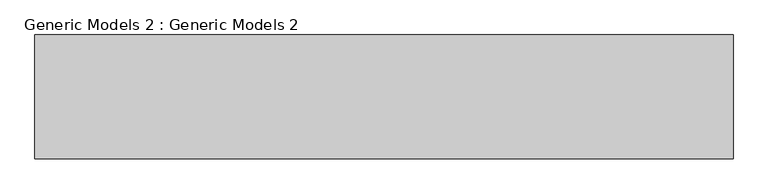
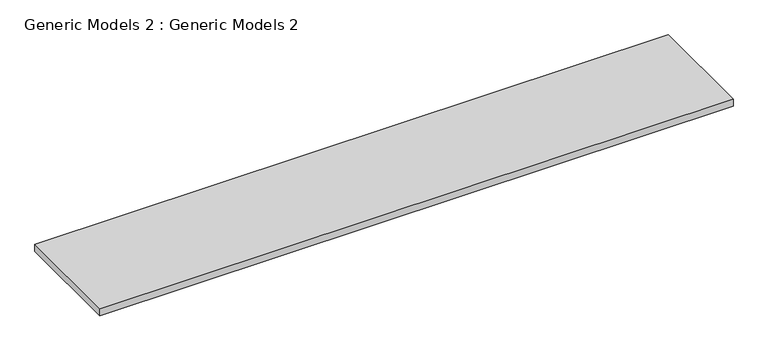
"""IFC4 building model written with IfcOpenShell, lengths in millimetres: proxy geometry, Generic Models 2 : Generic Models 2."""

from ifc_helpers import new_model, si_unit, origin, origin_with_axes, place, context, project, spatial, polyline, outline, extrude, source, transform, mapped, element, save


def generic_models_2_generic_models_2_d48e4085(model_context):
    return source(origin(), model_context, "Body", "SweptSolid", [
        extrude(outline(polyline([(-3802.4859258, -14004.7876618), (-16223.0859258, -14004.7876618), (-16223.0859258, -11801.0777232), (-3802.4859258, -11801.0777232), (-3802.4859258, -14004.7876618)])), origin_with_axes(), (0.0, 0.0, 1.0), 146.3632195),
    ])


if __name__ == "__main__":
    model = new_model("IFC4")
    model_context = context("Model", 3, world=origin())
    ifc_project = project(units=[si_unit("LENGTHUNIT", "METRE", prefix="MILLI")], contexts=[model_context])
    site = spatial("IfcSite", under=ifc_project)
    building = spatial("IfcBuilding", under=site)
    placement = place(None, origin())
    generic_models_2_generic_models_2_shape = generic_models_2_generic_models_2_d48e4085(model_context)
    element("IfcBuildingElementProxy", 1, Name="Generic Models 2 : Generic Models 2", ObjectType="Generic Models 2 : Generic Models 2", at=placement, inside=building, context=model_context, shape_type="MappedRepresentation", body=[
        mapped(generic_models_2_generic_models_2_shape, transform((0.0, 0.0, 0.0), x_axis=(1.0, 0.0, 0.0), y_axis=(0.0, 1.0, 0.0), z_axis=(0.0, 0.0, 1.0))),
    ])
    save(model, "model.ifc")
